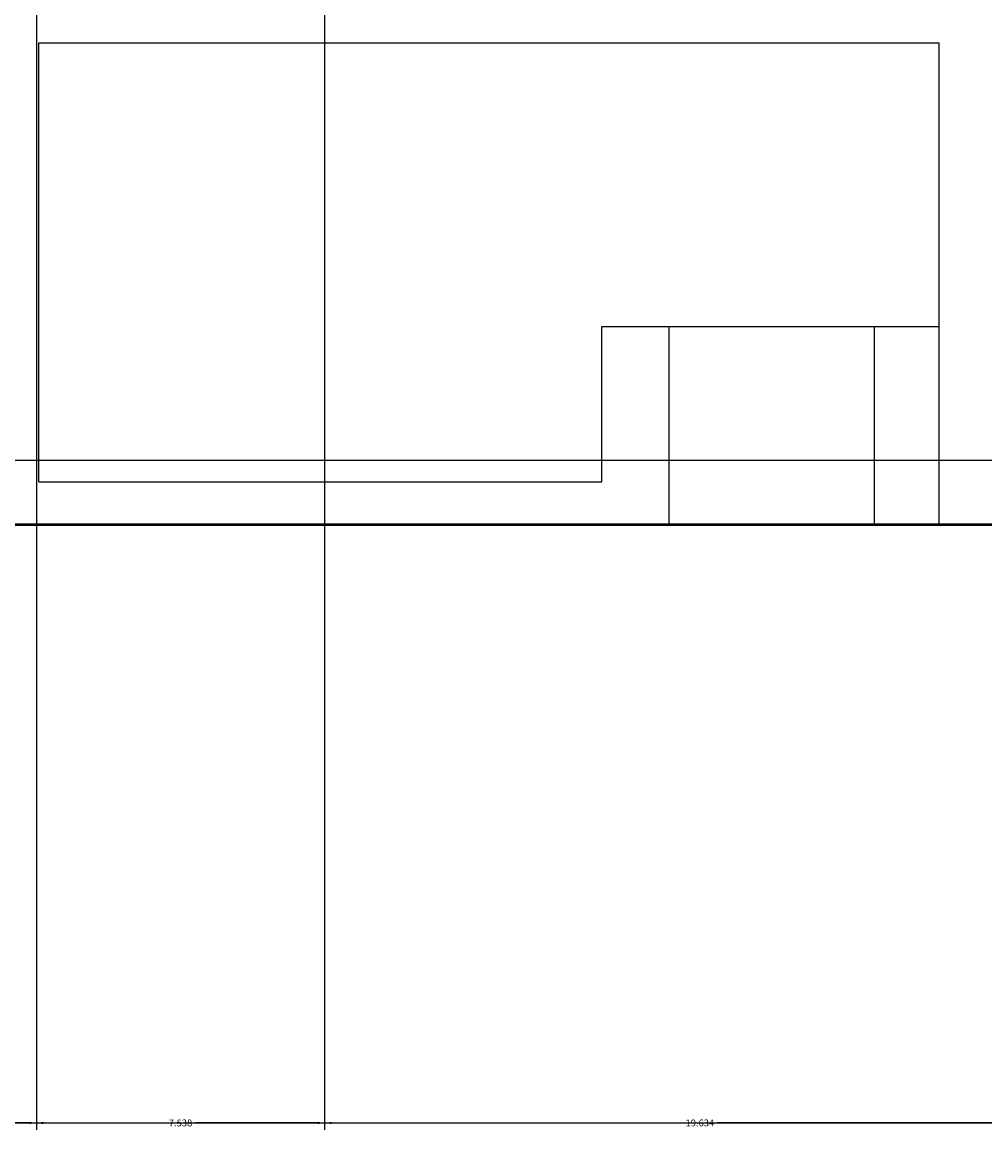
# Model space of a CAD drawing. Units: inches. Extents: x -117 to 121, y -77 to 40.
# Tile 5 of 45: x -73 to -48, y -77 to -48. Entities that reach past the tile are written whole.
import ezdxf

# ---------------------------------------------------------------- set-up
doc = ezdxf.new("R2010")
doc.units = ezdxf.units.IN
doc.header["$MEASUREMENT"] = 0
for name, color, linetype, lineweight in [('A-ANNO-DIMS', 2, 'Continuous', 18), ('A-ELEV', 7, 'Continuous', 25), ('A-ELEV-GRND', 7, 'Continuous', 50)]:
    doc.layers.add(name, color=color, linetype=linetype, lineweight=lineweight)
doc.styles.get("Standard").update_dxf_attribs({"font": 'arial.ttf'})
doc.dimstyles.get("Standard").update_dxf_attribs({"dimtxt": 0.18, "dimasz": 0.18, "dimexe": 0.18, "dimexo": 0.0625, "dimgap": 0.09, "dimtad": 0, "dimtih": 1, "dimtoh": 1, "dimdec": 4, "dimzin": 0, "dimdsep": 46, "dimtxsty": 'Standard', "dimcen": 0.09, "dimadec": 0, "dimazin": 0, "dimtfac": 1, "dimtdec": 4, "dimtofl": 0, "dimtmove": 0, "dimatfit": 3, "dimfxl": 1, "dimtolj": 1, "dimtzin": 0, "dimarcsym": 0})

# ---------------------------------------------------------------- blocks, each defined once
blk = doc.blocks.new('*D7')
at = {"layer": 'A-ANNO-DIMS', "color": 0, "lineweight": -2, "transparency": 16777216}
for p, q in [((-77.763, -61.431), (-77.763, -77.193)), ((90.549, -61.438), (90.549, -77.193)), ((-77.583, -77.013), (6.008, -77.013)), ((90.369, -77.013), (6.778, -77.013))]:
    blk.add_line(p, q, dxfattribs=at)
at = {"layer": 'A-ANNO-DIMS', "color": 0, "transparency": 16777216}
for points in [[(-77.583, -76.983), (-77.583, -77.043), (-77.763, -77.013)], [(90.369, -76.983), (90.369, -77.043), (90.549, -77.013)]]:
    blk.add_solid(points, dxfattribs=at)
at = {"layer": 'Defpoints', "color": 0, "transparency": 16777216}
for p in [(-77.763, -61.369), (90.549, -61.376), (90.549, -77.013)]:
    blk.add_point(p, dxfattribs=at)
at = {"layer": 'A-ANNO-DIMS', "color": 0, "transparency": 16777216, "insert": (6.393, -77.013), "char_height": 0.18, "attachment_point": 5}
blk.add_mtext('\\A1;168.3', dxfattribs=at)
blk = doc.blocks.new('*D13')
at = {"layer": 'A-ANNO-DIMS', "color": 0, "lineweight": -2, "transparency": 16777216}
for p, q in [((-2.663, 27.063), (-117.024, 27.063)), ((-116.844, 26.883), (-116.844, -16.974)), ((-116.844, -61.196), (-116.844, -17.338)), ((-106.096, -61.376), (-117.024, -61.376))]:
    blk.add_line(p, q, dxfattribs=at)
at = {"layer": 'A-ANNO-DIMS', "color": 0, "transparency": 16777216}
for points in [[(-116.874, 26.883), (-116.814, 26.883), (-116.844, 27.063)], [(-116.874, -61.196), (-116.814, -61.196), (-116.844, -61.376)]]:
    blk.add_solid(points, dxfattribs=at)
at = {"layer": 'Defpoints', "color": 0, "transparency": 16777216}
for p in [(-2.6, 27.063), (-116.844, -61.376), (-106.034, -61.376)]:
    blk.add_point(p, dxfattribs=at)
at = {"layer": 'A-ANNO-DIMS', "color": 0, "transparency": 16777216, "insert": (-116.844, -17.156), "char_height": 0.18, "attachment_point": 5}
blk.add_mtext('\\A1;88.44', dxfattribs=at)
blk = doc.blocks.new('*D37')
at = {"layer": 'A-ANNO-DIMS', "color": 0, "lineweight": -2, "transparency": 16777216}
for p, q in [((-3.912, -45.613), (-117.024, -45.613)), ((-116.844, -45.793), (-116.844, -52.47)), ((-116.844, -59.512), (-116.844, -52.834)), ((-3.912, -59.692), (-117.024, -59.692))]:
    blk.add_line(p, q, dxfattribs=at)
at = {"layer": 'A-ANNO-DIMS', "color": 0, "transparency": 16777216}
for points in [[(-116.874, -45.793), (-116.814, -45.793), (-116.844, -45.613)], [(-116.874, -59.512), (-116.814, -59.512), (-116.844, -59.692)]]:
    blk.add_solid(points, dxfattribs=at)
at = {"layer": 'Defpoints', "color": 0, "transparency": 16777216}
for p in [(-116.844, -45.613), (-3.85, -45.613), (-3.85, -59.692)]:
    blk.add_point(p, dxfattribs=at)
at = {"layer": 'A-ANNO-DIMS', "color": 0, "transparency": 16777216, "insert": (-116.844, -52.652), "char_height": 0.18, "attachment_point": 5}
blk.add_mtext('\\A1;14.079', dxfattribs=at)
blk = doc.blocks.new('*D46')
at = {"layer": 'A-ANNO-DIMS', "color": 0, "lineweight": -2, "transparency": 16777216}
for p, q in [((-78.307, -39.778), (-78.307, -77.193)), ((-72.705, -39.778), (-72.705, -77.193)), ((-78.127, -77.013), (-75.882, -77.013)), ((-72.885, -77.013), (-75.13, -77.013))]:
    blk.add_line(p, q, dxfattribs=at)
at = {"layer": 'A-ANNO-DIMS', "color": 0, "transparency": 16777216}
for points in [[(-78.127, -76.983), (-78.127, -77.043), (-78.307, -77.013)], [(-72.885, -76.983), (-72.885, -77.043), (-72.705, -77.013)]]:
    blk.add_solid(points, dxfattribs=at)
at = {"layer": 'Defpoints', "color": 0, "transparency": 16777216}
for p in [(-78.307, -39.716), (-72.705, -39.716), (-72.705, -77.013)]:
    blk.add_point(p, dxfattribs=at)
at = {"layer": 'A-ANNO-DIMS', "color": 0, "transparency": 16777216, "insert": (-75.506, -77.013), "char_height": 0.18, "attachment_point": 5}
blk.add_mtext('\\A1;5.601', dxfattribs=at)
blk = doc.blocks.new('*D47')
at = {"layer": 'A-ANNO-DIMS', "color": 0, "lineweight": -2, "transparency": 16777216}
for p, q in [((-72.705, -39.778), (-72.705, -77.193)), ((-65.167, -39.778), (-65.167, -77.193)), ((-72.525, -77.013), (-69.329, -77.013)), ((-65.347, -77.013), (-68.543, -77.013))]:
    blk.add_line(p, q, dxfattribs=at)
at = {"layer": 'A-ANNO-DIMS', "color": 0, "transparency": 16777216}
for points in [[(-72.525, -76.983), (-72.525, -77.043), (-72.705, -77.013)], [(-65.347, -76.983), (-65.347, -77.043), (-65.167, -77.013)]]:
    blk.add_solid(points, dxfattribs=at)
at = {"layer": 'Defpoints', "color": 0, "transparency": 16777216}
for p in [(-72.705, -39.716), (-65.167, -39.716), (-65.167, -77.013)]:
    blk.add_point(p, dxfattribs=at)
at = {"layer": 'A-ANNO-DIMS', "color": 0, "transparency": 16777216, "insert": (-68.936, -77.013), "char_height": 0.18, "attachment_point": 5}
blk.add_mtext('\\A1;7.538', dxfattribs=at)
blk = doc.blocks.new('*D48')
at = {"layer": 'A-ANNO-DIMS', "color": 0, "lineweight": -2, "transparency": 16777216}
for p, q in [((-65.167, -39.778), (-65.167, -77.193)), ((-45.533, -39.778), (-45.533, -77.193)), ((-64.987, -77.013), (-55.805, -77.013)), ((-45.713, -77.013), (-54.895, -77.013))]:
    blk.add_line(p, q, dxfattribs=at)
at = {"layer": 'A-ANNO-DIMS', "color": 0, "transparency": 16777216}
for points in [[(-64.987, -76.983), (-64.987, -77.043), (-65.167, -77.013)], [(-45.713, -76.983), (-45.713, -77.043), (-45.533, -77.013)]]:
    blk.add_solid(points, dxfattribs=at)
at = {"layer": 'Defpoints', "color": 0, "transparency": 16777216}
for p in [(-65.167, -39.716), (-45.533, -39.716), (-45.533, -77.013)]:
    blk.add_point(p, dxfattribs=at)
at = {"layer": 'A-ANNO-DIMS', "color": 0, "transparency": 16777216, "insert": (-55.35, -77.013), "char_height": 0.18, "attachment_point": 5}
blk.add_mtext('\\A1;19.634', dxfattribs=at)

msp = doc.modelspace()

# ---------------------------------------------------------------- linework, layer by layer
at = {"layer": 'A-ELEV'}
for p, q in [((-72.6404, -60.2463), (-72.6404, -48.7698)), ((-72.6404, -48.7698), (-49.086, -48.7698)), ((-49.086, -61.3756), (-49.086, -48.7698)), ((-57.9161, -60.2463), (-57.9161, -56.186)), ((-57.9161, -56.186), (-49.086, -56.186)), ((-56.1486, -61.3756), (-56.1486, -56.186)), ((-50.7806, -61.3756), (-50.7806, -56.186)), ((-72.6404, -60.2463), (-57.9161, -60.2463))]:
    msp.add_line(p, q, dxfattribs=at)
at = {"layer": 'A-ELEV-GRND'}
msp.add_line((90.5486, -61.3756), (-87.9273, -61.3756), dxfattribs=at)

# ---------------------------------------------------------------- dimensions: what is measured, and where the dimension line sits
at = {"layer": 'A-ANNO-DIMS'}
for base, p1, p2, override, picture, middle in [((-116.8438, -61.3756), (-2.6001, 27.0634), (-106.0338, -61.3756), {"dimdec": 2, "dimlfac": 1, "dimrnd": 0, "dimzin": 0, "dimdsep": 46, "dimlunit": 2}, '*D13', (-116.8438, -17.1561)), ((-116.843772, -45.612514), (-3.849514, -59.692012), (-3.849514, -45.612514), {"dimdec": 3, "dimlfac": 1, "dimrnd": 0, "dimzin": 0, "dimdsep": 46, "dimlunit": 2}, '*D37', (-116.843772, -52.652263))]:
    dim = msp.add_linear_dim(base=base, p1=p1, p2=p2, angle=90, dimstyle='Standard', override=override, dxfattribs=at)
    dim.commit()
    dim.dimension.update_dxf_attribs({"geometry": picture, "text_midpoint": middle})
for base, p1, p2, override, picture, middle in [((-72.70528, -77.01347), (-78.30676, -39.71597), (-72.70528, -39.71597), {"dimdec": 3, "dimlfac": 1, "dimrnd": 0, "dimzin": 0, "dimdsep": 46, "dimlunit": 2}, '*D46', (-75.50602, -77.01347)), ((-65.1673, -77.0135), (-72.7053, -39.716), (-65.1673, -39.716), {"dimdec": 3, "dimlfac": 1, "dimrnd": 0, "dimzin": 0, "dimdsep": 46, "dimlunit": 2}, '*D47', (-68.9363, -77.0135)), ((-45.5331, -77.0135), (-65.1673, -39.716), (-45.5331, -39.716), {"dimdec": 3, "dimlfac": 1, "dimrnd": 0, "dimzin": 0, "dimdsep": 46, "dimlunit": 2}, '*D48', (-55.3502, -77.0135)), ((90.5486, -77.0135), (-77.7631, -61.3689), (90.5486, -61.3756), {"dimdec": 1, "dimlfac": 1, "dimrnd": 0, "dimzin": 0, "dimdsep": 46, "dimlunit": 2}, '*D7', (6.3928, -77.0135))]:
    dim = msp.add_linear_dim(base=base, p1=p1, p2=p2, dimstyle='Standard', override=override, dxfattribs=at)
    dim.commit()
    dim.dimension.update_dxf_attribs({"geometry": picture, "text_midpoint": middle})

doc.saveas('drawing.dxf')
